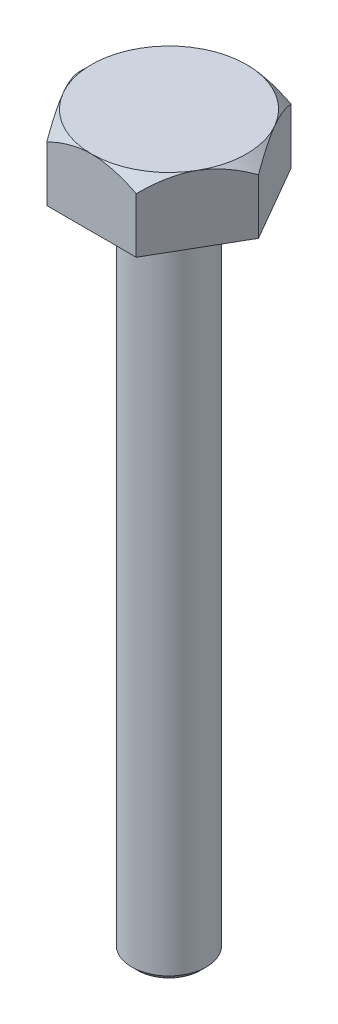
from build123d import *

# Parameters (mm, degrees)
HEX_HEAD_DEPTH                 = 45
HEAD_CHAMFER_PROFILE_OUTSIDE_W = 245.11
HEAD_CHAMFER_PROFILE_OUTSIDE_H = 229.022
HEAD_CHAMFER_PROFILE_OUTSIDE_R = 52
HEAD_TOP_CHAMFER_45DEG_DEPTH   = 45
HEAD_TOP_CHAMFER_45DEG_DRAFT   = -45
SHANK_PROFILE_50_R             = 25
SHANK_50X445_DEPTH             = 445
SHANK_END_CHAMFER_4X45DEG_SIZE = 4


with BuildPart() as part:
    # Hex Head Profile 104AF → Hex Head (new body)
    with BuildSketch(Plane(origin=(0, 0, 0), x_dir=(1, 0, 0), z_dir=(0, 1, 0))):
        Polygon((30.022213998, -52), (60.044427996, 0), (30.022213998, 52), (-30.022213998, 52), (-60.044427996, 0), (-30.022213998, -52), align=None)
    extrude(amount=HEX_HEAD_DEPTH)


with BuildPart() as head_top_chamfer_45deg_tool:
    # Head Chamfer Profile outside → Head Top Chamfer 45deg (with draft: the straight prism first)
    with BuildSketch(Plane(origin=(0, 45, 0), x_dir=(1, 0, 0), z_dir=(0, 1, 0))):
        Rectangle(HEAD_CHAMFER_PROFILE_OUTSIDE_W, HEAD_CHAMFER_PROFILE_OUTSIDE_H)
        Circle(HEAD_CHAMFER_PROFILE_OUTSIDE_R, mode=Mode.SUBTRACT)
    extrude(amount=-HEAD_TOP_CHAMFER_45DEG_DEPTH)
    # Head Top Chamfer 45deg: the draft: its side faces are tilted about the plane it starts from
    head_top_chamfer_45deg_sides = [head_top_chamfer_45deg_tool.faces().sort_by_distance(p)[0] for p in [
        (0, 22.5, 114.511),
        (122.555, 22.5, 0),
        (0, 22.5, -114.511),
        (-122.555, 22.5, 0),
        (-52, 22.5, 0),
    ]]
    draft(head_top_chamfer_45deg_sides, Plane(origin=(0, 45, 0), x_dir=(1, 0, 0), z_dir=(0, 1, 0)), HEAD_TOP_CHAMFER_45DEG_DRAFT)


with BuildPart() as part_1:
    add(part.part)

    # Head Top Chamfer 45deg: cut by head_top_chamfer_45deg_tool
    add(head_top_chamfer_45deg_tool.part, mode=Mode.SUBTRACT)

    # Shank Profile Ø50 → Shank Ø50x445 (add)
    with BuildSketch(Plane.XZ):
        with Locations(Location((0, 0, 0), (0, 0, 270))):
            Circle(SHANK_PROFILE_50_R)
    extrude(amount=SHANK_50X445_DEPTH)

    # Shank End Chamfer 4x45deg
    shank_end_chamfer_4x45deg_edges = [part_1.edges().sort_by_distance(p)[0] for p in [
        (0, -445, 25),
    ]]
    chamfer(shank_end_chamfer_4x45deg_edges, length=SHANK_END_CHAMFER_4X45DEG_SIZE)


solid = part_1.part
